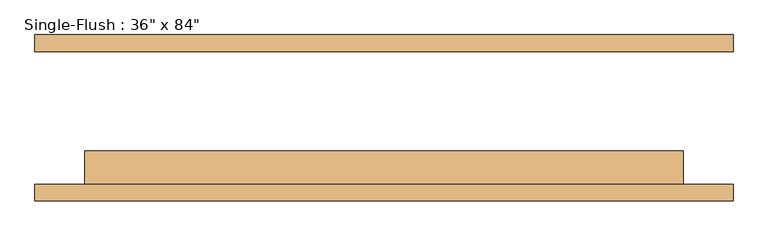
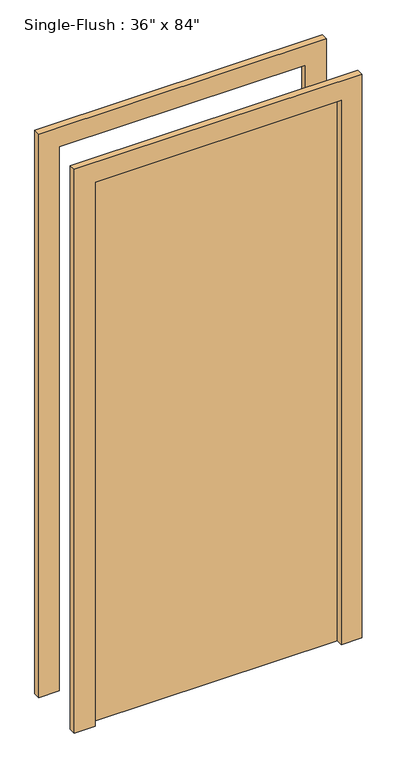
"""IFC4 building model written with IfcOpenShell, lengths in millimetres: door geometry."""

from ifc_helpers import new_model, si_unit, frame, origin, origin_with_axes, place, context, project, spatial, polyline, outline, extrude, source, transform, mapped, element, save


def door_719f80de(model_context):
    return source(origin(), model_context, "Body", "SweptSolid", [
        extrude(outline(polyline([(2209.8, -533.4), (0.0, -533.4), (0.0, -457.2), (2133.6, -457.2), (2133.6, 457.2), (0.0, 457.2), (0.0, 533.4), (2209.8, 533.4), (2209.8, -533.4)])), frame((0.0, -127.0, 0.0), z_axis=(0.0, 1.0, 0.0), x_axis=(0.0, 0.0, 1.0)), (0.0, 0.0, 1.0), 25.4),
        extrude(outline(polyline([(2209.8, 533.4), (2209.8, -533.4), (0.0, -533.4), (0.0, -457.2), (2133.6, -457.2), (2133.6, 457.2), (0.0, 457.2), (0.0, 533.4), (2209.8, 533.4)])), frame((0.0, 101.6, 0.0), z_axis=(0.0, 1.0, 0.0), x_axis=(0.0, 0.0, 1.0)), (0.0, 0.0, 1.0), 25.4),
        extrude(outline(polyline([(457.2, -50.8), (457.2, -101.6), (-457.2, -101.6), (-457.2, -50.8), (457.2, -50.8)])), origin_with_axes(), (0.0, 0.0, 1.0), 2133.6),
    ])


if __name__ == "__main__":
    model = new_model("IFC4")
    model_context = context("Model", 3, world=origin())
    ifc_project = project(units=[si_unit("LENGTHUNIT", "METRE", prefix="MILLI")], contexts=[model_context])
    site = spatial("IfcSite", under=ifc_project)
    building = spatial("IfcBuilding", under=site)
    placement = place(None, origin())
    door_shape = door_719f80de(model_context)
    element("IfcDoor", 1, ObjectType="Single-Flush : 36\" x 84\"", at=placement, inside=building, context=model_context, shape_type="MappedRepresentation", body=[
        mapped(door_shape, transform((0.0, 0.0, 0.0), x_axis=(1.0, 0.0, 0.0), y_axis=(0.0, 1.0, 0.0), z_axis=(0.0, 0.0, 1.0))),
    ])
    save(model, "model.ifc")

# Revit data of these elements
# Type "Single-Flush : 36\" x 84\""
#   Type Mark = "1"
#   Construction Type Id = "MDOOR"
#   Assembly Code = "C1020"
#   Analytic Construction = "Metal"
#   Thickness = 0' - 2"
#   Heat Transfer Coefficient (U) = 0.651978 BTU/(h·ft²·°F)
#   Height = 7' - 0"
#   Trim Projection Ext = 0' - 1"
#   Trim Projection Int = 0' - 1"
#   Trim Width = 0' - 3"
#   Width = 3' - 0"
#   Define Thermal Properties by = 1
#   Door Material = Door - Panel
#   Frame Material = Door - Frame
#   Visual Light Transmittance = 0
#   Solar Heat Gain Coefficient = 0
#   Function = (empty or 0)
#   Wall Closure = (empty or 0)
# Element 1 (IfcDoor, "Single-Flush : 36\" x 84\"")
#   Materials on its faces: "Door - Frame", "Door - Panel"
# Materials
#   "Door - Panel": class "Wood", colour RGB 210 159 95, transparency 0
#   "Door - Frame": colour RGB 118 70 51, transparency 0
